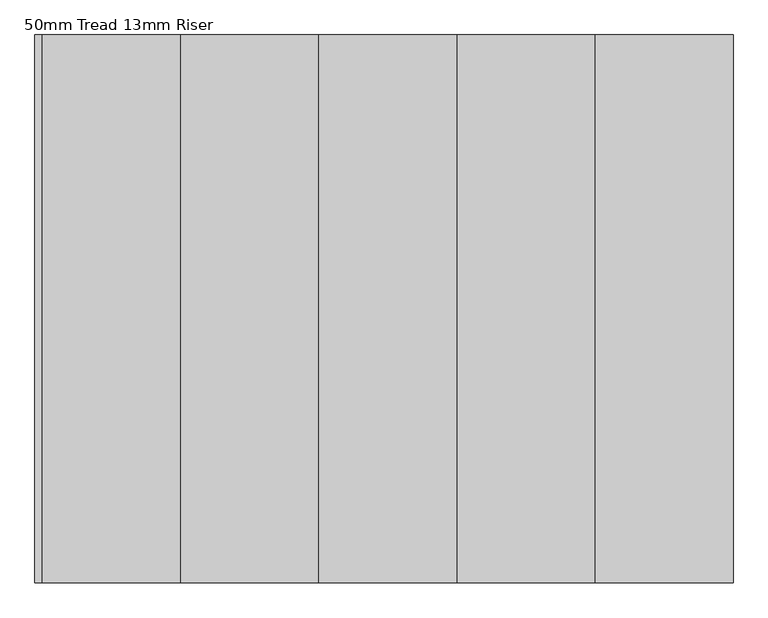
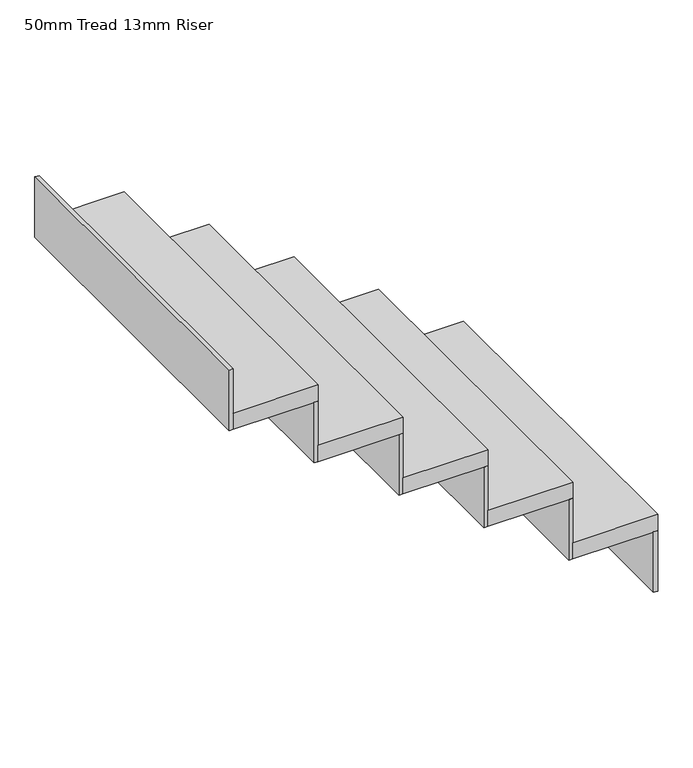
"""IFC4 building model written with IfcOpenShell, lengths in millimetres: stair flight geometry, 50mm Tread 13mm Riser."""

from ifc_helpers import new_model, si_unit, frame, origin, place, context, project, spatial, polyline, outline, extrude, source, transform, mapped, element, save


def stair_flight_50mm_tread_13mm_riser_ab1ff6a1(model_context):
    return source(origin(), model_context, "Body", "SweptSolid", [
        extrude(outline(polyline([(-10480.6794909, -3260.5618509), (-10468.1794909, -3260.5618509), (-10468.1794909, -4251.1618509), (-10480.6794909, -4251.1618509), (-10480.6794909, -3260.5618509)])), frame((0.0, 0.0, 2020.8470588), z_axis=(0.0, 0.0, 1.0), x_axis=(1.0, 0.0, 0.0)), (0.0, 0.0, 1.0), 188.2588235),
        extrude(outline(polyline([(-10718.1794909, -4251.1618509), (-10718.1794909, -3260.5618509), (-10468.1794909, -3260.5618509), (-10468.1794909, -4251.1618509), (-10718.1794909, -4251.1618509)])), frame((0.0, 0.0, 2209.1058824), z_axis=(0.0, 0.0, 1.0), x_axis=(1.0, 0.0, 0.0)), (0.0, 0.0, 1.0), 50.0),
        extrude(outline(polyline([(-10730.6794909, -3260.5618509), (-10718.1794909, -3260.5618509), (-10718.1794909, -4251.1618509), (-10730.6794909, -4251.1618509), (-10730.6794909, -3260.5618509)])), frame((0.0, 0.0, 2209.1058824), z_axis=(0.0, 0.0, 1.0), x_axis=(1.0, 0.0, 0.0)), (0.0, 0.0, 1.0), 188.2588235),
        extrude(outline(polyline([(-10968.1794909, -4251.1618509), (-10968.1794909, -3260.5618509), (-10718.1794909, -3260.5618509), (-10718.1794909, -4251.1618509), (-10968.1794909, -4251.1618509)])), frame((0.0, 0.0, 2397.3647059), z_axis=(0.0, 0.0, 1.0), x_axis=(1.0, 0.0, 0.0)), (0.0, 0.0, 1.0), 50.0),
        extrude(outline(polyline([(-10980.6794909, -3260.5618509), (-10968.1794909, -3260.5618509), (-10968.1794909, -4251.1618509), (-10980.6794909, -4251.1618509), (-10980.6794909, -3260.5618509)])), frame((0.0, 0.0, 2397.3647059), z_axis=(0.0, 0.0, 1.0), x_axis=(1.0, 0.0, 0.0)), (0.0, 0.0, 1.0), 188.2588235),
        extrude(outline(polyline([(-11218.1794909, -4251.1618509), (-11218.1794909, -3260.5618509), (-10968.1794909, -3260.5618509), (-10968.1794909, -4251.1618509), (-11218.1794909, -4251.1618509)])), frame((0.0, 0.0, 2585.6235294), z_axis=(0.0, 0.0, 1.0), x_axis=(1.0, 0.0, 0.0)), (0.0, 0.0, 1.0), 50.0),
        extrude(outline(polyline([(-11230.6794909, -3260.5618509), (-11218.1794909, -3260.5618509), (-11218.1794909, -4251.1618509), (-11230.6794909, -4251.1618509), (-11230.6794909, -3260.5618509)])), frame((0.0, 0.0, 2585.6235294), z_axis=(0.0, 0.0, 1.0), x_axis=(1.0, 0.0, 0.0)), (0.0, 0.0, 1.0), 188.2588235),
        extrude(outline(polyline([(-11468.1794909, -4251.1618509), (-11468.1794909, -3260.5618509), (-11218.1794909, -3260.5618509), (-11218.1794909, -4251.1618509), (-11468.1794909, -4251.1618509)])), frame((0.0, 0.0, 2773.8823529), z_axis=(0.0, 0.0, 1.0), x_axis=(1.0, 0.0, 0.0)), (0.0, 0.0, 1.0), 50.0),
        extrude(outline(polyline([(-11480.6794909, -3260.5618509), (-11468.1794909, -3260.5618509), (-11468.1794909, -4251.1618509), (-11480.6794909, -4251.1618509), (-11480.6794909, -3260.5618509)])), frame((0.0, 0.0, 2773.8823529), z_axis=(0.0, 0.0, 1.0), x_axis=(1.0, 0.0, 0.0)), (0.0, 0.0, 1.0), 188.2588235),
        extrude(outline(polyline([(-11730.6794909, -3260.5618509), (-11718.1794909, -3260.5618509), (-11718.1794909, -4251.1618509), (-11730.6794909, -4251.1618509), (-11730.6794909, -3260.5618509)])), frame((0.0, 0.0, 2962.1411765), z_axis=(0.0, 0.0, 1.0), x_axis=(1.0, 0.0, 0.0)), (0.0, 0.0, 1.0), 188.2588235),
        extrude(outline(polyline([(-11718.1794909, -4251.1618509), (-11718.1794909, -3260.5618509), (-11468.1794909, -3260.5618509), (-11468.1794909, -4251.1618509), (-11718.1794909, -4251.1618509)])), frame((0.0, 0.0, 2962.1411765), z_axis=(0.0, 0.0, 1.0), x_axis=(1.0, 0.0, 0.0)), (0.0, 0.0, 1.0), 50.0),
    ])


if __name__ == "__main__":
    model = new_model("IFC4")
    model_context = context("Model", 3, world=origin())
    ifc_project = project(units=[si_unit("LENGTHUNIT", "METRE", prefix="MILLI")], contexts=[model_context])
    site = spatial("IfcSite", under=ifc_project)
    building = spatial("IfcBuilding", under=site)
    placement = place(None, origin())
    stair_flight_50mm_tread_13mm_riser_shape = stair_flight_50mm_tread_13mm_riser_ab1ff6a1(model_context)
    element("IfcStairFlight", 1, ObjectType="50mm Tread 13mm Riser", at=placement, inside=building, context=model_context, shape_type="MappedRepresentation", body=[
        mapped(stair_flight_50mm_tread_13mm_riser_shape, transform((0.0, 0.0, 0.0), x_axis=(1.0, 0.0, 0.0), y_axis=(0.0, 1.0, 0.0), z_axis=(0.0, 0.0, 1.0))),
    ])
    save(model, "model.ifc")
